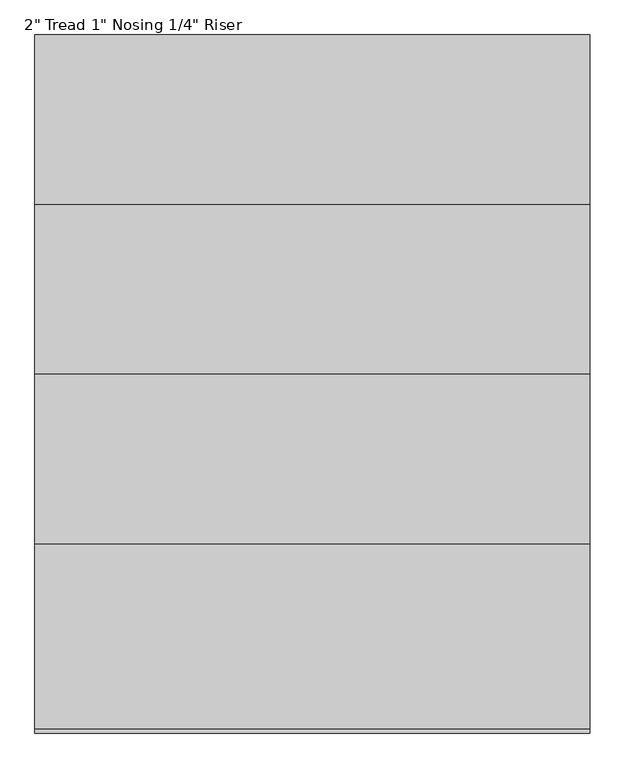
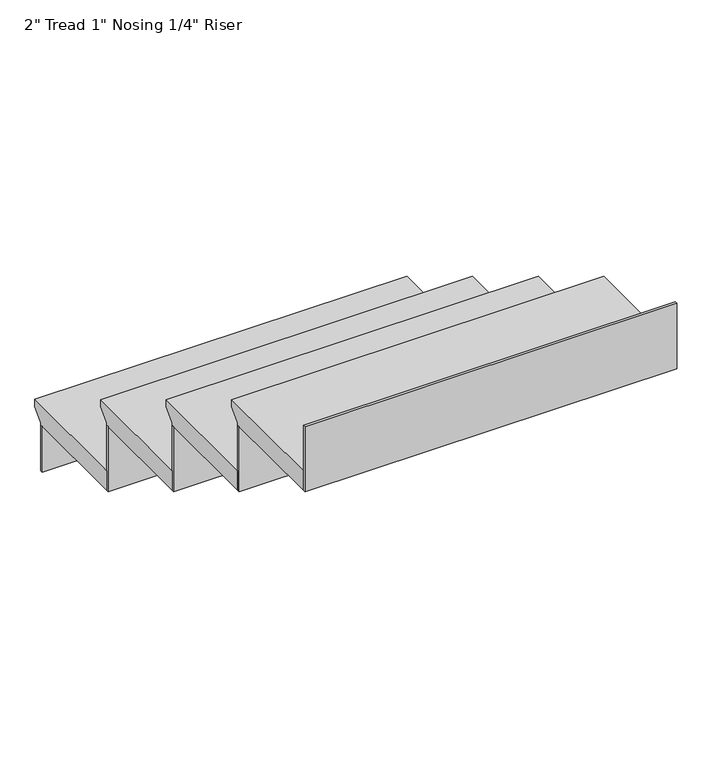
"""IFC4 building model written with IfcOpenShell, lengths in millimetres: stair flight geometry."""

from ifc_helpers import new_model, si_unit, origin, place, context, project, spatial, faceted_brep, source, transform, mapped, element, save


def stair_flight_15cb6ebf(model_context):
    return source(origin(), model_context, "Body", "Brep", [
        faceted_brep([(2695.3430349, 4115.4555142, 4383.6166667), (2695.3430349, 4115.4555142, 4402.6666667), (3609.7430349, 4115.4555142, 4402.6666667), (3609.7430349, 4115.4555142, 4383.6166667), (2695.3430349, 4090.0555142, 4358.2166667), (3609.7430349, 4090.0555142, 4358.2166667), (2695.3430349, 3810.6555142, 4402.6666667), (3609.7430349, 3810.6555142, 4402.6666667), (3609.7430349, 4090.0555142, 4351.8666667), (3609.7430349, 3810.6555142, 4351.8666667), (2695.3430349, 3810.6555142, 4351.8666667), (2695.3430349, 4090.0555142, 4351.8666667)], [[[0, 1, 2, 3]], [[4, 0, 3, 5]], [[2, 1, 6, 7]], [[8, 9, 10, 11]], [[2, 7, 9, 8, 5, 3]], [[8, 11, 4, 5]], [[6, 1, 0, 4, 11, 10]], [[7, 6, 10, 9]]]),
        faceted_brep([(2695.3430349, 4090.0555142, 4351.8666667), (2695.3430349, 4090.0555142, 4233.3333333), (2695.3430349, 4083.7055142, 4233.3333333), (2695.3430349, 4083.7055142, 4351.8666667), (3609.7430349, 4090.0555142, 4351.8666667), (3609.7430349, 4083.7055142, 4351.8666667), (3609.7430349, 4083.7055142, 4233.3333333), (3609.7430349, 4090.0555142, 4233.3333333)], [[[0, 1, 2, 3]], [[4, 5, 6, 7]], [[1, 0, 4, 7]], [[2, 1, 7, 6]], [[3, 2, 6, 5]], [[0, 3, 5, 4]]]),
        faceted_brep([(2695.3430349, 3810.6555142, 4521.2), (2695.3430349, 3810.6555142, 4351.8666667), (2695.3430349, 3804.3055142, 4351.8666667), (2695.3430349, 3804.3055142, 4521.2), (3609.7430349, 3810.6555142, 4521.2), (3609.7430349, 3804.3055142, 4521.2), (3609.7430349, 3804.3055142, 4351.8666667), (3609.7430349, 3810.6555142, 4351.8666667)], [[[0, 1, 2, 3]], [[4, 5, 6, 7]], [[1, 0, 4, 7]], [[2, 1, 7, 6]], [[3, 2, 6, 5]], [[0, 3, 5, 4]]]),
        faceted_brep([(3609.7430349, 3836.0555142, 4572.0), (2695.3430349, 3836.0555142, 4572.0), (2695.3430349, 3531.2555142, 4572.0), (3609.7430349, 3531.2555142, 4572.0), (3609.7430349, 3810.6555142, 4521.2), (3609.7430349, 3531.2555142, 4521.2), (2695.3430349, 3531.2555142, 4521.2), (2695.3430349, 3810.6555142, 4521.2), (3609.7430349, 3810.6555142, 4527.55), (3609.7430349, 3836.0555142, 4552.95), (2695.3430349, 3810.6555142, 4527.55), (2695.3430349, 3836.0555142, 4552.95)], [[[0, 1, 2, 3]], [[4, 5, 6, 7]], [[0, 3, 5, 4, 8, 9]], [[4, 7, 10, 8]], [[2, 1, 11, 10, 7, 6]], [[3, 2, 6, 5]], [[11, 1, 0, 9]], [[10, 11, 9, 8]]]),
        faceted_brep([(2695.3430349, 3531.2555142, 4690.5333333), (2695.3430349, 3531.2555142, 4521.2), (2695.3430349, 3524.9055142, 4521.2), (2695.3430349, 3524.9055142, 4690.5333333), (3609.7430349, 3531.2555142, 4690.5333333), (3609.7430349, 3524.9055142, 4690.5333333), (3609.7430349, 3524.9055142, 4521.2), (3609.7430349, 3531.2555142, 4521.2)], [[[0, 1, 2, 3]], [[4, 5, 6, 7]], [[1, 0, 4, 7]], [[2, 1, 7, 6]], [[3, 2, 6, 5]], [[0, 3, 5, 4]]]),
        faceted_brep([(3609.7430349, 3556.6555142, 4741.3333333), (2695.3430349, 3556.6555142, 4741.3333333), (2695.3430349, 3251.8555142, 4741.3333333), (3609.7430349, 3251.8555142, 4741.3333333), (3609.7430349, 3531.2555142, 4690.5333333), (3609.7430349, 3251.8555142, 4690.5333333), (2695.3430349, 3251.8555142, 4690.5333333), (2695.3430349, 3531.2555142, 4690.5333333), (3609.7430349, 3531.2555142, 4696.8833333), (3609.7430349, 3556.6555142, 4722.2833333), (2695.3430349, 3531.2555142, 4696.8833333), (2695.3430349, 3556.6555142, 4722.2833333)], [[[0, 1, 2, 3]], [[4, 5, 6, 7]], [[0, 3, 5, 4, 8, 9]], [[4, 7, 10, 8]], [[2, 1, 11, 10, 7, 6]], [[3, 2, 6, 5]], [[11, 1, 0, 9]], [[10, 11, 9, 8]]]),
        faceted_brep([(2695.3430349, 2972.4555142, 5029.2), (2695.3430349, 2972.4555142, 4859.8666667), (2695.3430349, 2966.1055142, 4859.8666667), (2695.3430349, 2966.1055142, 5029.2), (3609.7430349, 2972.4555142, 5029.2), (3609.7430349, 2966.1055142, 5029.2), (3609.7430349, 2966.1055142, 4859.8666667), (3609.7430349, 2972.4555142, 4859.8666667)], [[[0, 1, 2, 3]], [[4, 5, 6, 7]], [[1, 0, 4, 7]], [[2, 1, 7, 6]], [[3, 2, 6, 5]], [[0, 3, 5, 4]]]),
        faceted_brep([(2695.3430349, 3251.8555142, 4859.8666667), (2695.3430349, 3251.8555142, 4690.5333333), (2695.3430349, 3245.5055142, 4690.5333333), (2695.3430349, 3245.5055142, 4859.8666667), (3609.7430349, 3251.8555142, 4859.8666667), (3609.7430349, 3245.5055142, 4859.8666667), (3609.7430349, 3245.5055142, 4690.5333333), (3609.7430349, 3251.8555142, 4690.5333333)], [[[0, 1, 2, 3]], [[4, 5, 6, 7]], [[1, 0, 4, 7]], [[2, 1, 7, 6]], [[3, 2, 6, 5]], [[0, 3, 5, 4]]]),
        faceted_brep([(3609.7430349, 2972.4555142, 4910.6666667), (3609.7430349, 2997.8555142, 4910.6666667), (3609.7430349, 3277.2555142, 4910.6666667), (2695.3430349, 3277.2555142, 4910.6666667), (2695.3430349, 2972.4555142, 4910.6666667), (3609.7430349, 2997.8555142, 4859.8666667), (3609.7430349, 2972.4555142, 4859.8666667), (2695.3430349, 2972.4555142, 4859.8666667), (2695.3430349, 3251.8555142, 4859.8666667), (3609.7430349, 3251.8555142, 4859.8666667), (3609.7430349, 3251.8555142, 4866.2166667), (3609.7430349, 3277.2555142, 4891.6166667), (2695.3430349, 3251.8555142, 4866.2166667), (2695.3430349, 3277.2555142, 4891.6166667)], [[[0, 1, 2, 3, 4]], [[5, 6, 7, 8, 9]], [[1, 0, 6, 5]], [[2, 1, 5, 9, 10, 11]], [[9, 8, 12, 10]], [[4, 3, 13, 12, 8, 7]], [[0, 4, 7, 6]], [[13, 3, 2, 11]], [[12, 13, 11, 10]]]),
    ])


if __name__ == "__main__":
    model = new_model("IFC4")
    model_context = context("Model", 3, world=origin())
    ifc_project = project(units=[si_unit("LENGTHUNIT", "METRE", prefix="MILLI")], contexts=[model_context])
    site = spatial("IfcSite", under=ifc_project)
    building = spatial("IfcBuilding", under=site)
    placement = place(None, origin())
    stair_flight_shape = stair_flight_15cb6ebf(model_context)
    element("IfcStairFlight", 1, ObjectType="2\" Tread 1\" Nosing 1/4\" Riser", at=placement, inside=building, context=model_context, shape_type="MappedRepresentation", body=[
        mapped(stair_flight_shape, transform((0.0, 0.0, 0.0), x_axis=(1.0, 0.0, 0.0), y_axis=(0.0, 1.0, 0.0), z_axis=(0.0, 0.0, 1.0))),
    ])
    save(model, "model.ifc")
